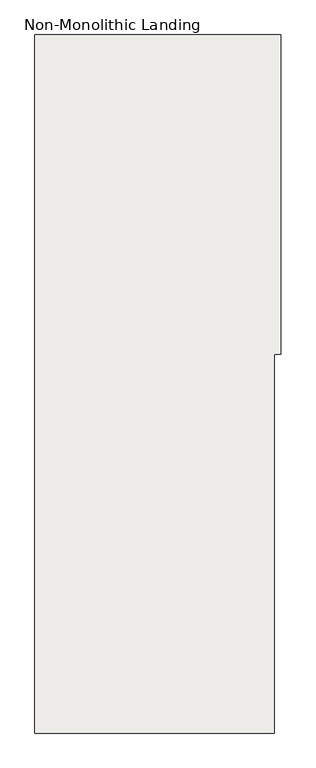
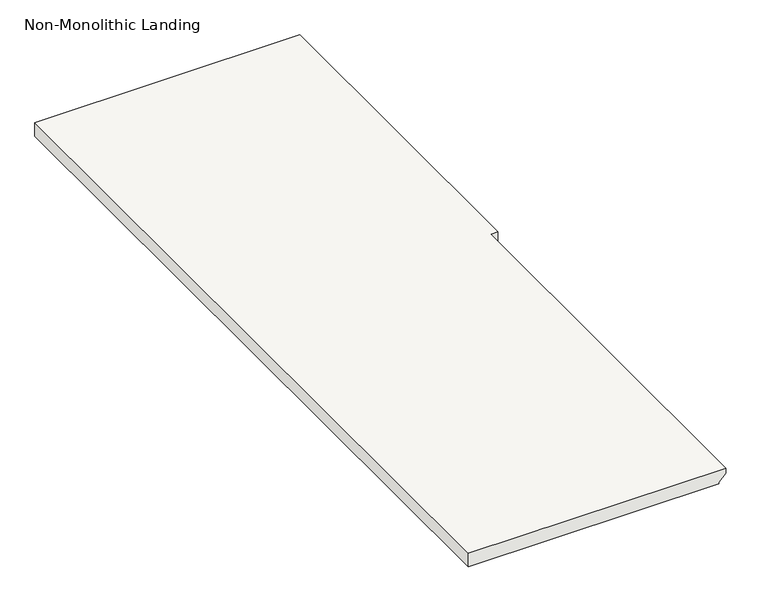
"""IFC4 building model written with IfcOpenShell, lengths in millimetres: slab geometry, Non-Monolithic Landing."""

from ifc_helpers import new_model, si_unit, origin, place, context, project, spatial, faceted_brep, source, transform, mapped, element, save


def non_monolithic_landing_a6573d81(model_context):
    return source(origin(), model_context, "Body", "Brep", [
        faceted_brep([(-8124.0791271, 5014.1953048, 1581.15), (-8149.4791271, 5014.1953048, 1555.75), (-8149.4791271, 6233.3953048, 1555.75), (-8124.0791271, 6233.3953048, 1581.15), (-8124.0791271, 6461.9953048, 1600.2), (-8098.6791271, 6461.9953048, 1600.2), (-8098.6791271, 7681.1953048, 1600.2), (-8124.0791271, 7681.1953048, 1600.2), (-9038.4791271, 7681.1953048, 1600.2), (-9038.4791271, 5014.1953048, 1600.2), (-8124.0791271, 5014.1953048, 1600.2), (-8149.4791271, 6233.3953048, 1549.4), (-8149.4791271, 5014.1953048, 1549.4), (-9038.4791271, 5014.1953048, 1549.4), (-9038.4791271, 7681.1953048, 1549.4), (-8124.0791271, 7681.1953048, 1549.4), (-8098.6791271, 7681.1953048, 1549.4), (-8098.6791271, 6461.9953048, 1549.4), (-8124.0791271, 6461.9953048, 1549.4), (-8124.0791271, 6233.3953048, 1549.4)], [[[0, 1, 2, 3]], [[4, 5, 6, 7, 8, 9, 10]], [[11, 12, 13, 14, 15, 16, 17, 18, 19]], [[12, 11, 2, 1]], [[11, 19, 3, 2]], [[4, 10, 0, 3, 19, 18]], [[5, 4, 18, 17]], [[6, 5, 17, 16]], [[7, 6, 16, 15]], [[8, 7, 15, 14]], [[9, 8, 14, 13]], [[10, 9, 13, 12, 1, 0]]]),
    ])


if __name__ == "__main__":
    model = new_model("IFC4")
    model_context = context("Model", 3, world=origin())
    ifc_project = project(units=[si_unit("LENGTHUNIT", "METRE", prefix="MILLI")], contexts=[model_context])
    site = spatial("IfcSite", under=ifc_project)
    building = spatial("IfcBuilding", under=site)
    placement = place(None, origin())
    non_monolithic_landing_shape = non_monolithic_landing_a6573d81(model_context)
    element("IfcSlab", 1, ObjectType="Non-Monolithic Landing", at=placement, inside=building, context=model_context, shape_type="MappedRepresentation", body=[
        mapped(non_monolithic_landing_shape, transform((0.0, 0.0, 0.0), x_axis=(1.0, 0.0, 0.0), y_axis=(0.0, 1.0, 0.0), z_axis=(0.0, 0.0, 1.0))),
    ])
    save(model, "model.ifc")
